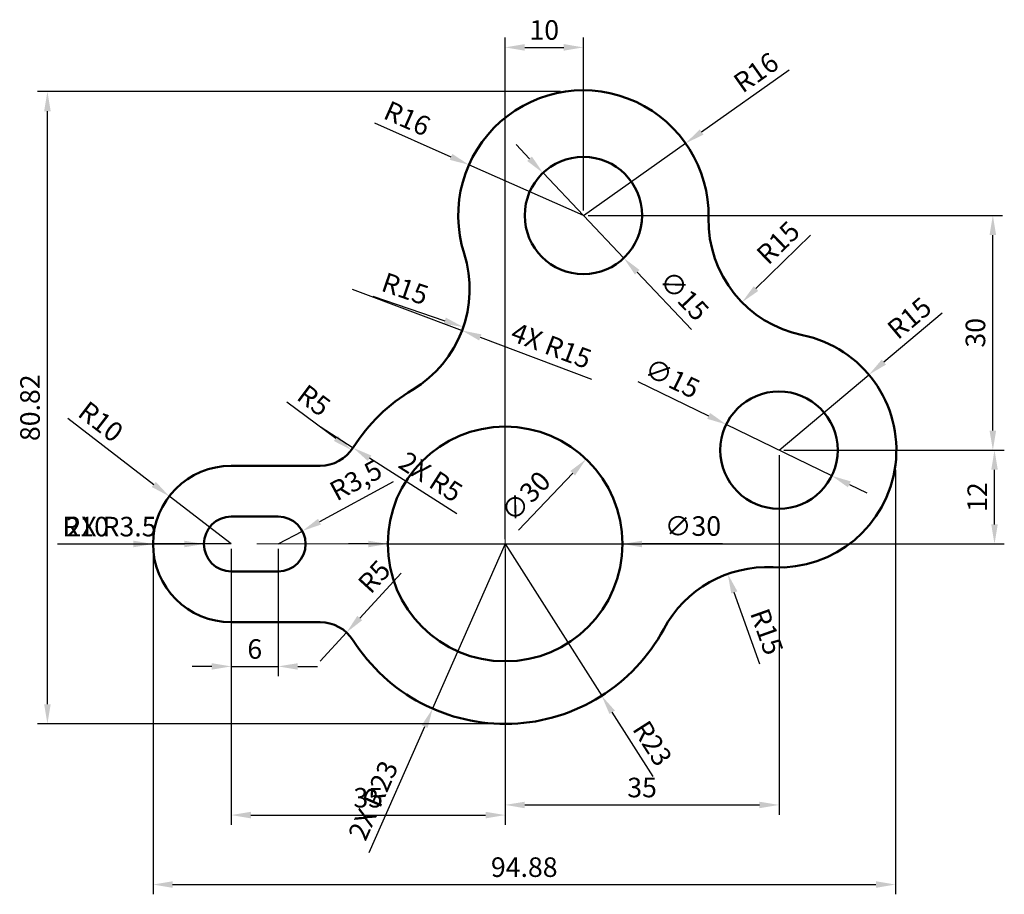
# Model space of a CAD drawing. Units: millimetres. Extents: x 3208 to 3333, y 1294 to 1406.
import ezdxf

# ---------------------------------------------------------------- set-up
doc = ezdxf.new("R2010")
doc.units = ezdxf.units.MM
doc.linetypes.add('CENTER', pattern=[50.8, 31.75, -6.35, 6.35, -6.35])
for name, color, linetype, lineweight in [('M-CNTR', 6, 'CENTER', 18), ('M-DIMS', 40, 'Continuous', 25), ('M-OUTL', 7, 'Continuous', 50)]:
    doc.layers.add(name, color=color, linetype=linetype, lineweight=lineweight)
doc.styles.get("Standard").update_dxf_attribs({"font": 'arial.ttf'})
doc.dimstyles.new('ISO-25', dxfattribs={"dimtxt": 2.5, "dimasz": 2.5, "dimexe": 1.25, "dimexo": 0.625, "dimtad": 1, "dimtxsty": 'Standard', "dimcen": 2.5, "dimadec": 0, "dimazin": 0, "dimtfac": 1, "dimtmove": 0, "dimatfit": 3, "dimfxl": 1, "dimarcsym": 0})

# ---------------------------------------------------------------- blocks, each defined once
blk = doc.blocks.new('*D1')
at = {"layer": 'Defpoints', "color": 0, "transparency": 16777216}
for p in [(3234.67, 1338.92), (3240.67, 1338.92), (3240.67, 1323.27)]:
    blk.add_point(p, dxfattribs=at)
at = {"layer": 'M-DIMS', "color": 0, "lineweight": -2, "transparency": 16777216}
for p, q in [((3234.67, 1338.29), (3234.67, 1322.02)), ((3240.67, 1338.29), (3240.67, 1322.02)), ((3232.17, 1323.27), (3229.67, 1323.27)), ((3234.67, 1323.27), (3240.67, 1323.27)), ((3243.17, 1323.27), (3245.67, 1323.27))]:
    blk.add_line(p, q, dxfattribs=at)
at = {"layer": 'M-DIMS', "color": 0, "transparency": 16777216}
for points in [[(3232.17, 1323.68), (3232.17, 1322.85), (3234.67, 1323.27)], [(3243.17, 1323.68), (3243.17, 1322.85), (3240.67, 1323.27)]]:
    blk.add_solid(points, dxfattribs=at)
at = {"layer": 'M-DIMS', "color": 0, "transparency": 16777216, "insert": (3237.67, 1325.17), "char_height": 2.5, "attachment_point": 5}
blk.add_mtext('6', dxfattribs=at)
blk = doc.blocks.new('*D2')
at = {"layer": 'Defpoints', "color": 0, "transparency": 16777216}
for p in [(3234.67, 1338.92), (3269.67, 1338.92), (3269.67, 1304.26)]:
    blk.add_point(p, dxfattribs=at)
at = {"layer": 'M-DIMS', "color": 0, "lineweight": -2, "transparency": 16777216}
for p, q in [((3234.67, 1338.29), (3234.67, 1303.01)), ((3269.67, 1338.29), (3269.67, 1303.01)), ((3237.17, 1304.26), (3267.17, 1304.26))]:
    blk.add_line(p, q, dxfattribs=at)
at = {"layer": 'M-DIMS', "color": 0, "transparency": 16777216}
for points in [[(3237.17, 1304.68), (3237.17, 1303.84), (3234.67, 1304.26)], [(3267.17, 1304.68), (3267.17, 1303.84), (3269.67, 1304.26)]]:
    blk.add_solid(points, dxfattribs=at)
at = {"layer": 'M-DIMS', "color": 0, "transparency": 16777216, "insert": (3252.17, 1306.16), "char_height": 2.5, "attachment_point": 5}
blk.add_mtext('35', dxfattribs=at)
blk = doc.blocks.new('*D3')
at = {"layer": 'Defpoints', "color": 0, "transparency": 16777216}
for p in [(3304.67, 1350.92), (3269.67, 1338.92), (3304.67, 1305.56)]:
    blk.add_point(p, dxfattribs=at)
at = {"layer": 'M-DIMS', "color": 0, "lineweight": -2, "transparency": 16777216}
for p, q in [((3304.67, 1350.29), (3304.67, 1304.31)), ((3269.67, 1338.29), (3269.67, 1304.31)), ((3272.17, 1305.56), (3302.17, 1305.56))]:
    blk.add_line(p, q, dxfattribs=at)
at = {"layer": 'M-DIMS', "color": 0, "transparency": 16777216}
for points in [[(3272.17, 1305.97), (3272.17, 1305.14), (3269.67, 1305.56)], [(3302.17, 1305.97), (3302.17, 1305.14), (3304.67, 1305.56)]]:
    blk.add_solid(points, dxfattribs=at)
at = {"layer": 'M-DIMS', "color": 0, "transparency": 16777216, "insert": (3287.17, 1307.46), "char_height": 2.5, "attachment_point": 5}
blk.add_mtext('35', dxfattribs=at)
blk = doc.blocks.new('*D4')
at = {"layer": 'Defpoints', "color": 0, "transparency": 16777216}
for p in [(3304.67, 1350.92), (3332.21, 1350.92), (3269.67, 1338.92)]:
    blk.add_point(p, dxfattribs=at)
at = {"layer": 'M-DIMS', "color": 0, "lineweight": -2, "transparency": 16777216}
for p, q in [((3305.29, 1350.92), (3333.46, 1350.92)), ((3332.21, 1341.42), (3332.21, 1348.42)), ((3270.29, 1338.92), (3333.46, 1338.92))]:
    blk.add_line(p, q, dxfattribs=at)
at = {"layer": 'M-DIMS', "color": 0, "transparency": 16777216}
for points in [[(3331.8, 1348.42), (3332.63, 1348.42), (3332.21, 1350.92)], [(3331.8, 1341.42), (3332.63, 1341.42), (3332.21, 1338.92)]]:
    blk.add_solid(points, dxfattribs=at)
at = {"layer": 'M-DIMS', "color": 0, "transparency": 16777216, "insert": (3330.33, 1344.92), "char_height": 2.5, "attachment_point": 5, "rotation": 90}
blk.add_mtext('12', dxfattribs=at)
blk = doc.blocks.new('*D5')
at = {"layer": 'Defpoints', "color": 0, "transparency": 16777216}
for p in [(3279.67, 1380.92), (3332, 1380.92), (3304.67, 1350.92)]:
    blk.add_point(p, dxfattribs=at)
at = {"layer": 'M-DIMS', "color": 0, "lineweight": -2, "transparency": 16777216}
for p, q in [((3280.29, 1380.92), (3333.25, 1380.92)), ((3332, 1353.42), (3332, 1378.42)), ((3305.29, 1350.92), (3333.25, 1350.92))]:
    blk.add_line(p, q, dxfattribs=at)
at = {"layer": 'M-DIMS', "color": 0, "transparency": 16777216}
for points in [[(3331.58, 1378.42), (3332.42, 1378.42), (3332, 1380.92)], [(3331.58, 1353.42), (3332.42, 1353.42), (3332, 1350.92)]]:
    blk.add_solid(points, dxfattribs=at)
at = {"layer": 'M-DIMS', "color": 0, "transparency": 16777216, "insert": (3330.1, 1365.92), "char_height": 2.5, "attachment_point": 5, "rotation": 90}
blk.add_mtext('30', dxfattribs=at)
blk = doc.blocks.new('*D6')
at = {"layer": 'Defpoints', "color": 0, "transparency": 16777216}
for p in [(3279.67, 1402.41), (3279.67, 1380.92), (3269.67, 1338.92)]:
    blk.add_point(p, dxfattribs=at)
at = {"layer": 'M-DIMS', "color": 0, "lineweight": -2, "transparency": 16777216}
for p, q in [((3269.67, 1339.54), (3269.67, 1403.66)), ((3279.67, 1381.54), (3279.67, 1403.66)), ((3272.17, 1402.41), (3277.17, 1402.41))]:
    blk.add_line(p, q, dxfattribs=at)
at = {"layer": 'M-DIMS', "color": 0, "transparency": 16777216}
for points in [[(3272.17, 1402.83), (3272.17, 1401.99), (3269.67, 1402.41)], [(3277.17, 1402.83), (3277.17, 1401.99), (3279.67, 1402.41)]]:
    blk.add_solid(points, dxfattribs=at)
at = {"layer": 'M-DIMS', "color": 0, "transparency": 16777216, "insert": (3274.67, 1404.31), "char_height": 2.5, "attachment_point": 5}
blk.add_mtext('10', dxfattribs=at)
blk = doc.blocks.new('*D7')
at = {"layer": 'Defpoints', "color": 0, "transparency": 16777216}
for p in [(3226.74, 1345.02), (3234.67, 1338.92)]:
    blk.add_point(p, dxfattribs=at)
at = {"layer": 'M-DIMS', "color": 0, "lineweight": -2, "transparency": 16777216}
for p, q in [((3213.78, 1354.99), (3224.76, 1346.54)), ((3234.67, 1338.92), (3226.74, 1345.02))]:
    blk.add_line(p, q, dxfattribs=at)
at = {"layer": 'M-DIMS', "color": 0, "transparency": 16777216}
blk.add_solid([(3225.02, 1346.87), (3224.51, 1346.21), (3226.74, 1345.02)], dxfattribs=at)
at = {"layer": 'M-DIMS', "color": 0, "transparency": 16777216, "insert": (3217.8, 1354.3), "char_height": 2.5, "attachment_point": 5, "rotation": 322.4196}
blk.add_mtext('R10', dxfattribs=at)
blk = doc.blocks.new('*D8')
at = {"layer": 'Defpoints', "color": 0, "transparency": 16777216}
for p in [(3246.03, 1353.92), (3250.03, 1350.93)]:
    blk.add_point(p, dxfattribs=at)
at = {"layer": 'M-DIMS', "color": 0, "lineweight": -2, "transparency": 16777216}
blk.add_line((3241.78, 1357.09), (3248.03, 1352.43), dxfattribs=at)
at = {"layer": 'M-DIMS', "color": 0, "transparency": 16777216}
blk.add_solid([(3248.28, 1352.76), (3247.78, 1352.09), (3250.03, 1350.93)], dxfattribs=at)
at = {"layer": 'M-DIMS', "color": 0, "transparency": 16777216, "insert": (3245.04, 1357.02), "char_height": 2.5, "attachment_point": 5, "rotation": 323.289}
blk.add_mtext('R5', dxfattribs=at)
blk = doc.blocks.new('*D9')
at = {"layer": 'Defpoints', "color": 0, "transparency": 16777216}
for p in [(3250.13, 1371.51), (3264.32, 1366.66)]:
    blk.add_point(p, dxfattribs=at)
at = {"layer": 'M-DIMS', "color": 0, "lineweight": -2, "transparency": 16777216}
blk.add_line((3252.74, 1370.62), (3261.96, 1367.47), dxfattribs=at)
at = {"layer": 'M-DIMS', "color": 0, "transparency": 16777216}
blk.add_solid([(3262.09, 1367.86), (3261.82, 1367.07), (3264.32, 1366.66)], dxfattribs=at)
at = {"layer": 'M-DIMS', "color": 0, "transparency": 16777216, "insert": (3256.78, 1371.25), "char_height": 2.5, "attachment_point": 5, "rotation": 341.1285}
blk.add_mtext('R15', dxfattribs=at)
blk = doc.blocks.new('*D10')
at = {"layer": 'Defpoints', "color": 0, "transparency": 16777216}
for p in [(3292.74, 1390.15), (3279.67, 1380.92)]:
    blk.add_point(p, dxfattribs=at)
at = {"layer": 'M-DIMS', "color": 0, "lineweight": -2, "transparency": 16777216}
for p, q in [((3305.96, 1399.48), (3294.78, 1391.59)), ((3279.67, 1380.92), (3292.74, 1390.15))]:
    blk.add_line(p, q, dxfattribs=at)
at = {"layer": 'M-DIMS', "color": 0, "transparency": 16777216}
blk.add_solid([(3294.54, 1391.93), (3295.02, 1391.25), (3292.74, 1390.15)], dxfattribs=at)
at = {"layer": 'M-DIMS', "color": 0, "transparency": 16777216, "insert": (3301.92, 1398.95), "char_height": 2.5, "attachment_point": 5, "rotation": 35.2159}
blk.add_mtext('R16', dxfattribs=at)
blk = doc.blocks.new('*D11')
at = {"layer": 'Defpoints', "color": 0, "transparency": 16777216}
for p in [(3310.66, 1380.31), (3299.94, 1369.82)]:
    blk.add_point(p, dxfattribs=at)
at = {"layer": 'M-DIMS', "color": 0, "lineweight": -2, "transparency": 16777216}
blk.add_line((3308.69, 1378.39), (3301.73, 1371.57), dxfattribs=at)
at = {"layer": 'M-DIMS', "color": 0, "transparency": 16777216}
blk.add_solid([(3301.44, 1371.87), (3302.02, 1371.27), (3299.94, 1369.82)], dxfattribs=at)
at = {"layer": 'M-DIMS', "color": 0, "transparency": 16777216, "insert": (3304.78, 1377.21), "char_height": 2.5, "attachment_point": 5, "rotation": 44.3907}
blk.add_mtext('R15', dxfattribs=at)
blk = doc.blocks.new('*D12')
at = {"layer": 'Defpoints', "color": 0, "transparency": 16777216}
for p in [(3316.16, 1360.56), (3304.67, 1350.92)]:
    blk.add_point(p, dxfattribs=at)
at = {"layer": 'M-DIMS', "color": 0, "lineweight": -2, "transparency": 16777216}
for p, q in [((3325.53, 1368.44), (3318.07, 1362.17)), ((3304.67, 1350.92), (3316.16, 1360.56))]:
    blk.add_line(p, q, dxfattribs=at)
at = {"layer": 'M-DIMS', "color": 0, "transparency": 16777216}
blk.add_solid([(3317.8, 1362.49), (3318.34, 1361.85), (3316.16, 1360.56)], dxfattribs=at)
at = {"layer": 'M-DIMS', "color": 0, "transparency": 16777216, "insert": (3321.54, 1367.56), "char_height": 2.5, "attachment_point": 5, "rotation": 40.0153}
blk.add_mtext('R15', dxfattribs=at)
blk = doc.blocks.new('*D13')
at = {"layer": 'Defpoints', "color": 0, "transparency": 16777216}
for p in [(3269.67, 1338.92), (3282.01, 1319.51)]:
    blk.add_point(p, dxfattribs=at)
at = {"layer": 'M-DIMS', "color": 0, "lineweight": -2, "transparency": 16777216}
for p, q in [((3269.67, 1338.92), (3282.01, 1319.51)), ((3288.57, 1309.19), (3283.35, 1317.4))]:
    blk.add_line(p, q, dxfattribs=at)
at = {"layer": 'M-DIMS', "color": 0, "transparency": 16777216}
blk.add_solid([(3283.7, 1317.62), (3283, 1317.18), (3282.01, 1319.51)], dxfattribs=at)
at = {"layer": 'M-DIMS', "color": 0, "transparency": 16777216, "insert": (3288.23, 1313.26), "char_height": 2.5, "attachment_point": 5, "rotation": 302.4424}
blk.add_mtext('R23', dxfattribs=at)
blk = doc.blocks.new('*D14')
at = {"layer": 'Defpoints', "color": 0, "transparency": 16777216}
for p in [(3298.12, 1335.09), (3303.16, 1320.96)]:
    blk.add_point(p, dxfattribs=at)
at = {"layer": 'M-DIMS', "color": 0, "lineweight": -2, "transparency": 16777216}
blk.add_line((3302.23, 1323.56), (3298.96, 1332.73), dxfattribs=at)
at = {"layer": 'M-DIMS', "color": 0, "transparency": 16777216}
blk.add_solid([(3299.35, 1332.87), (3298.57, 1332.59), (3298.12, 1335.09)], dxfattribs=at)
at = {"layer": 'M-DIMS', "color": 0, "transparency": 16777216, "insert": (3302.81, 1327.6), "char_height": 2.5, "attachment_point": 5, "rotation": 289.609}
blk.add_mtext('R15', dxfattribs=at)
blk = doc.blocks.new('*D15')
at = {"layer": 'Defpoints', "color": 0, "transparency": 16777216}
for p in [(3249.4, 1327.61), (3246.03, 1323.92)]:
    blk.add_point(p, dxfattribs=at)
at = {"layer": 'M-DIMS', "color": 0, "lineweight": -2, "transparency": 16777216}
for p, q in [((3256.36, 1335.21), (3251.09, 1329.45)), ((3246.03, 1323.92), (3249.4, 1327.61))]:
    blk.add_line(p, q, dxfattribs=at)
at = {"layer": 'M-DIMS', "color": 0, "transparency": 16777216}
blk.add_solid([(3250.78, 1329.73), (3251.4, 1329.17), (3249.4, 1327.61)], dxfattribs=at)
at = {"layer": 'M-DIMS', "color": 0, "transparency": 16777216, "insert": (3253.17, 1334.53), "char_height": 2.5, "attachment_point": 5, "rotation": 47.53}
blk.add_mtext('R5', dxfattribs=at)
blk = doc.blocks.new('*D16')
at = {"layer": 'Defpoints', "color": 0, "transparency": 16777216}
for p in [(3243.75, 1340.58), (3240.67, 1338.92)]:
    blk.add_point(p, dxfattribs=at)
at = {"layer": 'M-DIMS', "color": 0, "lineweight": -2, "transparency": 16777216}
for p, q in [((3255.37, 1346.87), (3245.95, 1341.77)), ((3240.67, 1338.92), (3243.75, 1340.58))]:
    blk.add_line(p, q, dxfattribs=at)
at = {"layer": 'M-DIMS', "color": 0, "transparency": 16777216}
blk.add_solid([(3245.75, 1342.14), (3246.14, 1341.41), (3243.75, 1340.58)], dxfattribs=at)
at = {"layer": 'M-DIMS', "color": 0, "transparency": 16777216, "insert": (3250.74, 1346.79), "char_height": 2.5, "attachment_point": 5, "rotation": 28.4124}
blk.add_mtext('R3,5', dxfattribs=at)
blk = doc.blocks.new('*D17')
at = {"layer": 'Defpoints', "color": 0, "transparency": 16777216}
for p in [(3280.02, 1349.77), (3259.31, 1328.07)]:
    blk.add_point(p, dxfattribs=at)
at = {"layer": 'M-DIMS', "color": 0, "lineweight": -2, "transparency": 16777216}
blk.add_line((3271.37, 1340.7), (3278.3, 1347.96), dxfattribs=at)
at = {"layer": 'M-DIMS', "color": 0, "transparency": 16777216}
blk.add_solid([(3278, 1348.25), (3278.6, 1347.68), (3280.02, 1349.77)], dxfattribs=at)
at = {"layer": 'M-DIMS', "color": 0, "transparency": 16777216, "insert": (3272.54, 1344.79), "char_height": 2.5, "attachment_point": 5, "rotation": 46.3399}
blk.add_mtext('∅30', dxfattribs=at)
blk = doc.blocks.new('*D18')
at = {"layer": 'Defpoints', "color": 0, "transparency": 16777216}
for p in [(3297.93, 1354.2), (3311.41, 1347.64)]:
    blk.add_point(p, dxfattribs=at)
at = {"layer": 'M-DIMS', "color": 0, "lineweight": -2, "transparency": 16777216}
for p, q in [((3286.62, 1359.7), (3295.68, 1355.3)), ((3311.41, 1347.64), (3297.93, 1354.2)), ((3313.66, 1346.54), (3315.91, 1345.45))]:
    blk.add_line(p, q, dxfattribs=at)
at = {"layer": 'M-DIMS', "color": 0, "transparency": 16777216}
for points in [[(3295.86, 1355.67), (3295.5, 1354.92), (3297.93, 1354.2)], [(3313.84, 1346.92), (3313.48, 1346.17), (3311.41, 1347.64)]]:
    blk.add_solid(points, dxfattribs=at)
at = {"layer": 'M-DIMS', "color": 0, "transparency": 16777216, "insert": (3290.89, 1359.82), "char_height": 2.5, "attachment_point": 5, "rotation": 334.0505}
blk.add_mtext('∅15', dxfattribs=at)
blk = doc.blocks.new('*D19')
at = {"layer": 'Defpoints', "color": 0, "transparency": 16777216}
for p in [(3274.51, 1386.36), (3284.83, 1375.48)]:
    blk.add_point(p, dxfattribs=at)
at = {"layer": 'M-DIMS', "color": 0, "lineweight": -2, "transparency": 16777216}
for p, q in [((3272.79, 1388.17), (3271.07, 1389.99)), ((3274.51, 1386.36), (3284.83, 1375.48)), ((3293.48, 1366.36), (3286.55, 1373.67))]:
    blk.add_line(p, q, dxfattribs=at)
at = {"layer": 'M-DIMS', "color": 0, "transparency": 16777216}
for points in [[(3273.09, 1388.46), (3272.48, 1387.89), (3274.51, 1386.36)], [(3286.85, 1373.95), (3286.25, 1373.38), (3284.83, 1375.48)]]:
    blk.add_solid(points, dxfattribs=at)
at = {"layer": 'M-DIMS', "color": 0, "transparency": 16777216, "insert": (3292.31, 1370.46), "char_height": 2.5, "attachment_point": 5, "rotation": 313.4949}
blk.add_mtext('∅15', dxfattribs=at)
blk = doc.blocks.new('HOLE-D15')
blk.add_circle((7.5, 7.5), 7.5)
blk = doc.blocks.new('*D21')
at = {"layer": 'Defpoints', "color": 0, "transparency": 16777216}
for p in [(3319.55, 1349.04), (3224.67, 1338.92), (3319.55, 1295.38)]:
    blk.add_point(p, dxfattribs=at)
at = {"layer": 'M-DIMS', "color": 0, "lineweight": -2, "transparency": 16777216}
for p, q in [((3319.55, 1348.41), (3319.55, 1294.13)), ((3224.67, 1338.29), (3224.67, 1294.13)), ((3227.17, 1295.38), (3317.05, 1295.38))]:
    blk.add_line(p, q, dxfattribs=at)
at = {"layer": 'M-DIMS', "color": 0, "transparency": 16777216}
for points in [[(3227.17, 1295.8), (3227.17, 1294.96), (3224.67, 1295.38)], [(3317.05, 1295.8), (3317.05, 1294.96), (3319.55, 1295.38)]]:
    blk.add_solid(points, dxfattribs=at)
at = {"layer": 'M-DIMS', "color": 0, "transparency": 16777216, "insert": (3272.11, 1297.28), "char_height": 2.5, "attachment_point": 5}
blk.add_mtext('94.88', dxfattribs=at)
blk = doc.blocks.new('*D22')
at = {"layer": 'Defpoints', "color": 0, "transparency": 16777216}
for p in [(3211.17, 1396.75), (3277.37, 1396.75), (3270.51, 1315.93)]:
    blk.add_point(p, dxfattribs=at)
at = {"layer": 'M-DIMS', "color": 0, "lineweight": -2, "transparency": 16777216}
for p, q in [((3276.74, 1396.75), (3209.92, 1396.75)), ((3211.17, 1318.43), (3211.17, 1394.25)), ((3269.88, 1315.93), (3209.92, 1315.93))]:
    blk.add_line(p, q, dxfattribs=at)
at = {"layer": 'M-DIMS', "color": 0, "transparency": 16777216}
for points in [[(3210.75, 1394.25), (3211.59, 1394.25), (3211.17, 1396.75)], [(3210.75, 1318.43), (3211.59, 1318.43), (3211.17, 1315.93)]]:
    blk.add_solid(points, dxfattribs=at)
at = {"layer": 'M-DIMS', "color": 0, "transparency": 16777216, "insert": (3209.27, 1356.34), "char_height": 2.5, "attachment_point": 5, "rotation": 90}
blk.add_mtext('80.82', dxfattribs=at)
blk = doc.blocks.new('*D23')
at = {"layer": 'Defpoints', "color": 0, "transparency": 16777216}
for p in [(3269.67, 1338.92), (3260.4, 1317.87)]:
    blk.add_point(p, dxfattribs=at)
at = {"layer": 'M-DIMS', "color": 0, "lineweight": -2, "transparency": 16777216}
for p, q in [((3269.67, 1338.92), (3260.4, 1317.87)), ((3252.29, 1299.46), (3259.39, 1315.58))]:
    blk.add_line(p, q, dxfattribs=at)
at = {"layer": 'M-DIMS', "color": 0, "transparency": 16777216}
blk.add_solid([(3259.01, 1315.75), (3259.77, 1315.41), (3260.4, 1317.87)], dxfattribs=at)
at = {"layer": 'M-DIMS', "color": 0, "transparency": 16777216, "insert": (3253.1, 1306.01), "char_height": 2.5, "attachment_point": 5, "rotation": 66.2335}
blk.add_mtext('2X R23', dxfattribs=at)
blk = doc.blocks.new('*D24')
at = {"layer": 'Defpoints', "color": 0, "transparency": 16777216}
for p in [(3265.04, 1387.4), (3279.67, 1380.92)]:
    blk.add_point(p, dxfattribs=at)
at = {"layer": 'M-DIMS', "color": 0, "lineweight": -2, "transparency": 16777216}
for p, q in [((3252.96, 1392.75), (3262.75, 1388.41)), ((3279.67, 1380.92), (3265.04, 1387.4))]:
    blk.add_line(p, q, dxfattribs=at)
at = {"layer": 'M-DIMS', "color": 0, "transparency": 16777216}
blk.add_solid([(3262.92, 1388.79), (3262.59, 1388.03), (3265.04, 1387.4)], dxfattribs=at)
at = {"layer": 'M-DIMS', "color": 0, "transparency": 16777216, "insert": (3257.03, 1393.03), "char_height": 2.5, "attachment_point": 5, "rotation": 336.1077}
blk.add_mtext('R16', dxfattribs=at)
blk = doc.blocks.new('*D25')
at = {"layer": 'Defpoints', "color": 0, "transparency": 16777216}
for p in [(3254.67, 1338.92), (3284.67, 1338.92)]:
    blk.add_point(p, dxfattribs=at)
at = {"layer": 'M-DIMS', "color": 0, "lineweight": -2, "transparency": 16777216}
for p, q in [((3252.17, 1338.92), (3249.67, 1338.92)), ((3254.67, 1338.92), (3284.67, 1338.92)), ((3297.44, 1338.92), (3287.17, 1338.92))]:
    blk.add_line(p, q, dxfattribs=at)
at = {"layer": 'M-DIMS', "color": 0, "transparency": 16777216}
for points in [[(3252.17, 1339.34), (3252.17, 1338.5), (3254.67, 1338.92)], [(3287.17, 1339.34), (3287.17, 1338.5), (3284.67, 1338.92)]]:
    blk.add_solid(points, dxfattribs=at)
at = {"layer": 'M-DIMS', "color": 0, "transparency": 16777216, "insert": (3293.67, 1340.89), "char_height": 2.5, "attachment_point": 5, "rotation": 0.0017}
blk.add_mtext('∅30', dxfattribs=at)
blk = doc.blocks.new('*D26')
at = {"layer": 'Defpoints', "color": 0, "transparency": 16777216}
for p in [(3250.13, 1371.51), (3264.16, 1366.21)]:
    blk.add_point(p, dxfattribs=at)
at = {"layer": 'M-DIMS', "color": 0, "lineweight": -2, "transparency": 16777216}
for p, q in [((3250.13, 1371.51), (3264.16, 1366.21)), ((3280.74, 1359.95), (3266.5, 1365.33))]:
    blk.add_line(p, q, dxfattribs=at)
at = {"layer": 'M-DIMS', "color": 0, "transparency": 16777216}
blk.add_solid([(3266.65, 1365.72), (3266.35, 1364.94), (3264.16, 1366.21)], dxfattribs=at)
at = {"layer": 'M-DIMS', "color": 0, "transparency": 16777216, "insert": (3275.46, 1363.98), "char_height": 2.5, "attachment_point": 5, "rotation": 339.3043}
blk.add_mtext('4X R15', dxfattribs=at)
blk = doc.blocks.new('*D27')
at = {"layer": 'Defpoints', "color": 0, "transparency": 16777216}
for p in [(3224.67, 1338.92), (3234.67, 1338.92)]:
    blk.add_point(p, dxfattribs=at)
at = {"layer": 'M-DIMS', "color": 0, "lineweight": -2, "transparency": 16777216}
for p, q in [((3212.45, 1338.92), (3222.17, 1338.92)), ((3234.67, 1338.92), (3224.67, 1338.92))]:
    blk.add_line(p, q, dxfattribs=at)
at = {"layer": 'M-DIMS', "color": 0, "transparency": 16777216}
blk.add_solid([(3222.17, 1339.34), (3222.17, 1338.5), (3224.67, 1338.92)], dxfattribs=at)
at = {"layer": 'M-DIMS', "color": 0, "transparency": 16777216, "insert": (3216.06, 1340.82), "char_height": 2.5, "attachment_point": 5, "rotation": 359.9975}
blk.add_mtext('R10', dxfattribs=at)
blk = doc.blocks.new('*D28')
at = {"layer": 'Defpoints', "color": 0, "transparency": 16777216}
for p in [(3246.03, 1353.92), (3250.24, 1351.22)]:
    blk.add_point(p, dxfattribs=at)
at = {"layer": 'M-DIMS', "color": 0, "lineweight": -2, "transparency": 16777216}
for p, q in [((3246.03, 1353.92), (3250.24, 1351.22)), ((3263.48, 1342.76), (3252.34, 1349.88))]:
    blk.add_line(p, q, dxfattribs=at)
at = {"layer": 'M-DIMS', "color": 0, "transparency": 16777216}
blk.add_solid([(3252.57, 1350.23), (3252.12, 1349.53), (3250.24, 1351.22)], dxfattribs=at)
at = {"layer": 'M-DIMS', "color": 0, "transparency": 16777216, "insert": (3259.99, 1347.24), "char_height": 2.5, "attachment_point": 5, "rotation": 327.3898}
blk.add_mtext('2X R5', dxfattribs=at)
blk = doc.blocks.new('*D29')
at = {"layer": 'Defpoints', "color": 0, "transparency": 16777216}
for p in [(3231.17, 1338.92), (3234.67, 1338.92)]:
    blk.add_point(p, dxfattribs=at)
at = {"layer": 'M-DIMS', "color": 0, "lineweight": -2, "transparency": 16777216}
for p, q in [((3212.54, 1338.92), (3228.67, 1338.92)), ((3234.67, 1338.92), (3231.17, 1338.92))]:
    blk.add_line(p, q, dxfattribs=at)
at = {"layer": 'M-DIMS', "color": 0, "transparency": 16777216}
blk.add_solid([(3228.67, 1339.34), (3228.67, 1338.5), (3231.17, 1338.92)], dxfattribs=at)
at = {"layer": 'M-DIMS', "color": 0, "transparency": 16777216, "insert": (3219.36, 1340.82), "char_height": 2.5, "attachment_point": 5, "rotation": 359.9928}
blk.add_mtext('2X R3.5', dxfattribs=at)

msp = doc.modelspace()

# ---------------------------------------------------------------- linework, layer by layer
at = {"layer": 'M-CNTR'}
for p, q in [((3269.669, 1359.449), (3269.669, 1308.882)), ((3269.669, 1338.92), (3234.669, 1338.92)), ((3269.669, 1338.92), (3304.669, 1338.92))]:
    msp.add_line(p, q, dxfattribs=at)
at = {"layer": 'M-OUTL'}
for p, q in [((3234.669, 1348.92), (3246.026, 1348.92)), ((3234.669, 1342.42), (3240.669, 1342.42)), ((3234.669, 1335.42), (3240.669, 1335.42)), ((3234.669, 1328.92), (3246.026, 1328.92))]:
    msp.add_line(p, q, dxfattribs=at)
msp.add_circle((3269.669, 1338.92), 15, dxfattribs=at)
for centre, radius, start, end in [((3279.669, 1380.92), 16, 358.88189, 197.66621), ((3310.663, 1380.315), 15, 178.88189, 258.47455), ((3250.131, 1371.512), 15, 300.94129, 17.66621), ((3304.669, 1350.92), 15, 267.10898, 78.47455), ((3269.669, 1338.92), 23, 120.94129, 147.60763), ((3246.026, 1353.92), 5, 270, 327.60763), ((3234.669, 1338.92), 10, 90, 270), ((3234.669, 1338.92), 3.5, 90, 270), ((3240.669, 1338.92), 3.5, 270, 90), ((3303.156, 1320.958), 15, 87.10898, 151.79163), ((3246.026, 1323.92), 5, 32.39237, 90), ((3269.669, 1338.92), 23, 212.39237, 331.79163)]:
    msp.add_arc(centre, radius, start, end, dxfattribs=at)

# ---------------------------------------------------------------- block references
for p in [(3272.169, 1373.42), (3297.169, 1343.42)]:
    msp.add_blockref('HOLE-D15', p, dxfattribs=at)

# ---------------------------------------------------------------- dimensions: what is measured, and where the dimension line sits
at = {"layer": 'M-DIMS'}
for base, p1, p2, override, picture, middle in [((3279.669, 1402.409), (3269.669, 1338.92), (3279.669, 1380.92), {"dimclrd": 0, "dimclre": 0, "dimclrt": 0}, '*D6', (3274.669, 1404.311)), ((3304.669, 1305.556), (3269.669, 1338.92), (3304.669, 1350.92), {"dimclrd": 0, "dimclre": 0, "dimclrt": 0}, '*D3', (3287.169, 1307.458)), ((3319.551, 1295.382), (3224.669, 1338.92), (3319.551, 1349.037), {"dimdec": 2, "dimlfac": 1, "dimrnd": 0, "dimzin": 0, "dimdsep": 46, "dimlunit": 2}, '*D21', (3272.11, 1297.283)), ((3240.669, 1323.267), (3234.669, 1338.92), (3240.669, 1338.92), {"dimclrd": 0, "dimclre": 0, "dimclrt": 0}, '*D1', (3237.669, 1325.168)), ((3269.669, 1304.26), (3234.669, 1338.92), (3269.669, 1338.92), {"dimclrd": 0, "dimclre": 0, "dimclrt": 0}, '*D2', (3252.169, 1306.162))]:
    dim = msp.add_linear_dim(base=base, p1=p1, p2=p2, dimstyle='ISO-25', override=override, dxfattribs=at)
    dim.commit()
    dim.dimension.update_dxf_attribs({"geometry": picture, "text_midpoint": middle})
for center, mpoint, override, picture, middle in [((3279.669, 1380.92), (3292.741, 1390.146), {"dimclrd": 0, "dimclre": 0, "dimclrt": 0}, '*D10', (3303.014, 1397.397)), ((3279.669, 1380.92), (3265.04, 1387.4), {"dimdec": 0, "dimlfac": 1, "dimrnd": 0, "dimzin": 0, "dimdsep": 46, "dimlunit": 2}, '*D24', (3256.263, 1391.288)), ((3310.663, 1380.315), (3299.945, 1369.821), {"dimclrd": 0, "dimclre": 0, "dimclrt": 0}, '*D11', (3306.105, 1375.852)), ((3250.131, 1371.512), (3264.325, 1366.66), {"dimclrd": 0, "dimclre": 0, "dimclrt": 0}, '*D9', (3256.167, 1369.449)), ((3246.026, 1353.92), (3250.034, 1350.931), {"dimclrd": 0, "dimclre": 0, "dimclrt": 0}, '*D8', (3243.902, 1355.504)), ((3234.669, 1338.92), (3226.744, 1345.018), {"dimclrd": 0, "dimclre": 0, "dimclrt": 0}, '*D7', (3216.64, 1352.794)), ((3303.156, 1320.958), (3298.122, 1335.088), {"dimclrd": 0, "dimclre": 0, "dimclrt": 0}, '*D14', (3301.015, 1326.967))]:
    dim = msp.add_radius_dim(center=center, mpoint=mpoint, dimstyle='ISO-25', override=override, dxfattribs=at)
    dim.commit()
    dim.dimension.update_dxf_attribs({"geometry": picture, "text_midpoint": middle, "dimtype": 164})
for base, p1, p2, override, picture, middle in [((3211.169, 1396.753), (3270.509, 1315.935), (3277.367, 1396.753), {"dimdec": 2, "dimlfac": 1, "dimrnd": 0, "dimzin": 0, "dimdsep": 46, "dimlunit": 2}, '*D22', (3209.268, 1356.344)), ((3332.002, 1380.92), (3304.669, 1350.92), (3279.669, 1380.92), {"dimclrd": 0, "dimclre": 0, "dimclrt": 0}, '*D5', (3330.099, 1365.92)), ((3332.215, 1350.92), (3269.669, 1338.92), (3304.669, 1350.92), {"dimclrd": 0, "dimclre": 0, "dimclrt": 0}, '*D4', (3330.335, 1344.92))]:
    dim = msp.add_linear_dim(base=base, p1=p1, p2=p2, angle=90, dimstyle='ISO-25', override=override, dxfattribs=at)
    dim.commit()
    dim.dimension.update_dxf_attribs({"geometry": picture, "text_midpoint": middle})
for p1, p2, picture, middle in [((3274.507, 1386.36), (3284.831, 1375.479), '*D19', (3292.308, 1370.463)), ((3311.413, 1347.638), (3297.925, 1354.201), '*D18', (3290.889, 1359.818))]:
    dim = msp.add_diameter_dim_2p(p1=p1, p2=p2, dimstyle='ISO-25', override={"dimclrd": 0, "dimclre": 0, "dimclrt": 0}, dxfattribs=at)
    dim.commit()
    dim.dimension.update_dxf_attribs({"geometry": picture, "text_midpoint": middle})
for center, mpoint, text, override, picture, middle in [((3250.131, 1371.512), (3264.163, 1366.211), '4X <>', {"dimdec": 0, "dimlfac": 1, "dimrnd": 0, "dimzin": 0, "dimdsep": 46, "dimlunit": 2}, '*D26', (3275.46, 1363.976)), ((3246.026, 1353.92), (3250.238, 1351.225), '2X <>', {"dimdec": 0, "dimlfac": 1, "dimrnd": 0, "dimzin": 0, "dimdsep": 46, "dimlunit": 2}, '*D28', (3259.987, 1347.245)), ((3234.669, 1338.92), (3231.169, 1338.92), '2X <>', {"dimdec": 1, "dimlfac": 1, "dimrnd": 0, "dimzin": 0, "dimdsep": 46, "dimlunit": 2}, '*D29', (3219.356, 1340.824))]:
    dim = msp.add_radius_dim(center=center, mpoint=mpoint, text=text, dimstyle='ISO-25', override=override, dxfattribs=at)
    dim.commit()
    dim.dimension.update_dxf_attribs({"geometry": picture, "text_midpoint": middle})
for center, mpoint, override, picture, middle in [((3304.669, 1350.92), (3316.157, 1360.564), {"dimclrd": 0, "dimclre": 0, "dimclrt": 0}, '*D12', (3321.538, 1367.564)), ((3240.669, 1338.92), (3243.748, 1340.585), {"dimclrd": 0, "dimclre": 0, "dimclrt": 0}, '*D16', (3250.745, 1346.789)), ((3234.669, 1338.92), (3224.669, 1338.92), {"dimdec": 0, "dimlfac": 1, "dimrnd": 0, "dimzin": 0, "dimdsep": 46, "dimlunit": 2}, '*D27', (3216.062, 1340.822)), ((3269.669, 1338.92), (3282.008, 1319.509), {"dimclrd": 0, "dimclre": 0, "dimclrt": 0}, '*D13', (3288.233, 1313.262)), ((3246.026, 1323.92), (3249.402, 1327.608), {"dimclrd": 0, "dimclre": 0, "dimclrt": 0}, '*D15', (3253.169, 1334.531))]:
    dim = msp.add_radius_dim(center=center, mpoint=mpoint, dimstyle='ISO-25', override=override, dxfattribs=at)
    dim.commit()
    dim.dimension.update_dxf_attribs({"geometry": picture, "text_midpoint": middle})
for p1, p2, override, picture, middle in [((3259.314, 1328.068), (3280.025, 1349.771), {"dimclrd": 0, "dimclre": 0, "dimclrt": 0}, '*D17', (3273.969, 1343.426)), ((3254.669, 1338.919), (3284.669, 1338.92), {"dimdec": 0, "dimlfac": 1, "dimrnd": 0, "dimzin": 0, "dimdsep": 46, "dimlunit": 2}, '*D25', (3293.669, 1338.92))]:
    dim = msp.add_diameter_dim_2p(p1=p1, p2=p2, dimstyle='ISO-25', override=override, dxfattribs=at)
    dim.commit()
    dim.dimension.update_dxf_attribs({"geometry": picture, "text_midpoint": middle, "dimtype": 163})
dim = msp.add_radius_dim(center=(3269.669, 1338.92), mpoint=(3260.4, 1317.87), text='2X <>', dimstyle='ISO-25', override={"dimdec": 0, "dimlfac": 1, "dimrnd": 0, "dimzin": 0, "dimdsep": 46, "dimlunit": 2}, dxfattribs=at)
dim.commit()
dim.dimension.update_dxf_attribs({"geometry": '*D23', "text_midpoint": (3254.838, 1305.24), "dimtype": 164})

doc.saveas('drawing.dxf')
